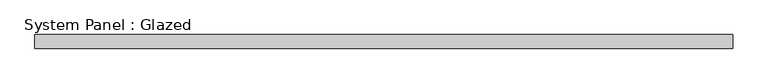
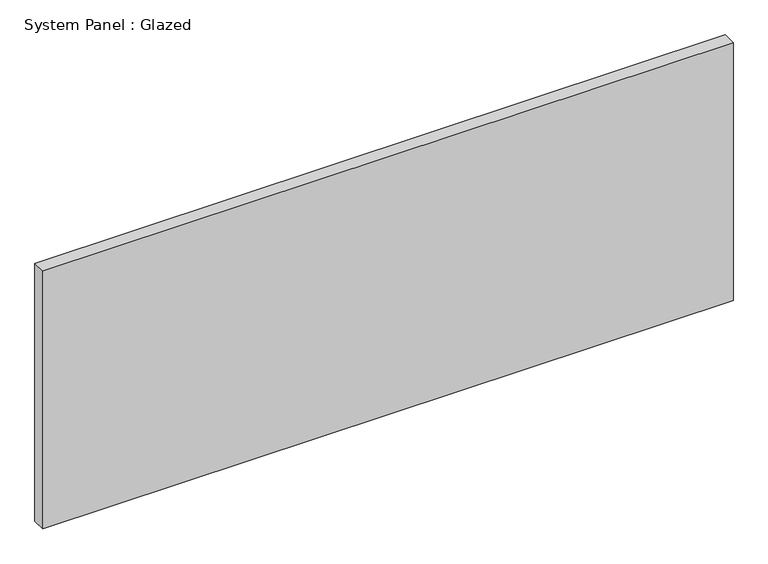
"""IFC4 building model written with IfcOpenShell, lengths in millimetres: plate geometry, System Panel : Glazed."""

from ifc_helpers import new_model, si_unit, origin, origin_with_axes, place, context, project, spatial, polyline, outline, extrude, source, transform, mapped, element, save


def system_panel_glazed_2e6a26f2(model_context):
    return source(origin(), model_context, "Body", "SweptSolid", [
        extrude(outline(polyline([(650.8750001, -44.45), (-650.8750001, -44.45), (-650.8750001, -19.05), (650.8750001, -19.05), (650.8750001, -44.45)])), origin_with_axes(), (0.0, 0.0, 1.0), 514.35),
    ])


if __name__ == "__main__":
    model = new_model("IFC4")
    model_context = context("Model", 3, world=origin())
    ifc_project = project(units=[si_unit("LENGTHUNIT", "METRE", prefix="MILLI")], contexts=[model_context])
    site = spatial("IfcSite", under=ifc_project)
    building = spatial("IfcBuilding", under=site)
    placement = place(None, origin())
    system_panel_glazed_shape = system_panel_glazed_2e6a26f2(model_context)
    element("IfcPlate", 1, ObjectType="System Panel : Glazed", at=placement, inside=building, context=model_context, shape_type="MappedRepresentation", body=[
        mapped(system_panel_glazed_shape, transform((0.0, 0.0, 0.0), x_axis=(1.0, 0.0, 0.0), y_axis=(0.0, 1.0, 0.0), z_axis=(0.0, 0.0, 1.0))),
    ])
    save(model, "model.ifc")

# Revit data of these elements
# Type "System Panel : Glazed"
#   Construction Type Id = "GSP4R"
#   Analytic Construction = "1/8 in Pilkington single glazing"
#   Visual Light Transmittance = 0.9
#   Solar Heat Gain Coefficient = 0.86
#   Heat Transfer Coefficient (U) = 1.18115 BTU/(h·ft²·°F)
#   Define Thermal Properties by = 1
# Element 1 (IfcPlate, "System Panel : Glazed")
#   Materials on its faces: "glass panel 223"
# Materials
#   "glass panel 223": class "Generic", colour RGB 120 120 120, transparency 0, Cost = 0
